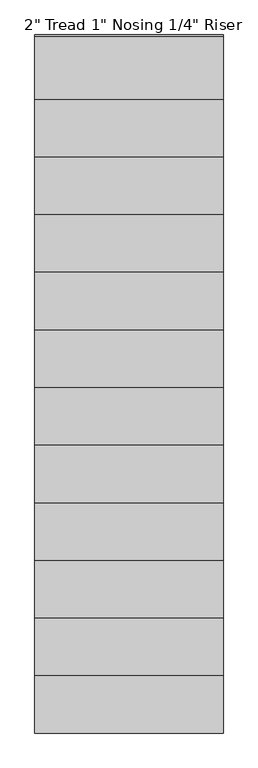
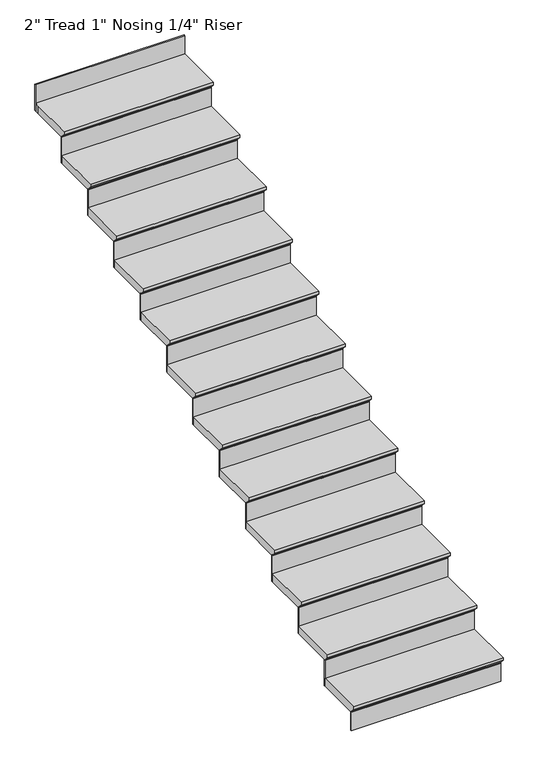
"""IFC4 building model written with IfcOpenShell, lengths in millimetres: stair flight geometry."""

from ifc_helpers import new_model, si_unit, origin, place, context, project, spatial, faceted_brep, source, transform, mapped, element, save


def stair_flight_770626d1(model_context):
    return source(origin(), model_context, "Body", "Brep", [
        faceted_brep([(-2703.0415084, 19841.9216096, 28432.9005799), (-2703.0415084, 19841.9216096, 28451.9505799), (-3617.4415084, 19841.9216096, 28451.9505799), (-3617.4415084, 19841.9216096, 28432.9005799), (-2703.0415084, 19867.3216096, 28407.5005799), (-3617.4415084, 19867.3216096, 28407.5005799), (-2703.0415084, 20146.7216096, 28451.9505799), (-3617.4415084, 20146.7216096, 28451.9505799), (-3617.4415084, 19867.3216096, 28401.1505799), (-3617.4415084, 20146.7216096, 28401.1505799), (-2703.0415084, 20146.7216096, 28401.1505799), (-2703.0415084, 19867.3216096, 28401.1505799)], [[[0, 1, 2, 3]], [[4, 0, 3, 5]], [[2, 1, 6, 7]], [[8, 9, 10, 11]], [[2, 7, 9, 8, 5, 3]], [[8, 11, 4, 5]], [[6, 1, 0, 4, 11, 10]], [[7, 6, 10, 9]]]),
        faceted_brep([(-2703.0415084, 19867.3216096, 28401.1505799), (-2703.0415084, 19867.3216096, 28282.6172466), (-2703.0415084, 19873.6716096, 28282.6172466), (-2703.0415084, 19873.6716096, 28401.1505799), (-3617.4415084, 19867.3216096, 28401.1505799), (-3617.4415084, 19873.6716096, 28401.1505799), (-3617.4415084, 19873.6716096, 28282.6172466), (-3617.4415084, 19867.3216096, 28282.6172466)], [[[0, 1, 2, 3]], [[4, 5, 6, 7]], [[1, 0, 4, 7]], [[2, 1, 7, 6]], [[3, 2, 6, 5]], [[0, 3, 5, 4]]]),
        faceted_brep([(-2703.0415084, 20146.7216096, 28570.4839133), (-2703.0415084, 20146.7216096, 28401.1505799), (-2703.0415084, 20153.0716096, 28401.1505799), (-2703.0415084, 20153.0716096, 28570.4839133), (-3617.4415084, 20146.7216096, 28570.4839133), (-3617.4415084, 20153.0716096, 28570.4839133), (-3617.4415084, 20153.0716096, 28401.1505799), (-3617.4415084, 20146.7216096, 28401.1505799)], [[[0, 1, 2, 3]], [[4, 5, 6, 7]], [[1, 0, 4, 7]], [[2, 1, 7, 6]], [[3, 2, 6, 5]], [[0, 3, 5, 4]]]),
        faceted_brep([(-3617.4415084, 20121.3216096, 28621.2839133), (-2703.0415084, 20121.3216096, 28621.2839133), (-2703.0415084, 20426.1216096, 28621.2839133), (-3617.4415084, 20426.1216096, 28621.2839133), (-3617.4415084, 20146.7216096, 28570.4839133), (-3617.4415084, 20426.1216096, 28570.4839133), (-2703.0415084, 20426.1216096, 28570.4839133), (-2703.0415084, 20146.7216096, 28570.4839133), (-3617.4415084, 20146.7216096, 28576.8339133), (-3617.4415084, 20121.3216096, 28602.2339133), (-2703.0415084, 20146.7216096, 28576.8339133), (-2703.0415084, 20121.3216096, 28602.2339133)], [[[0, 1, 2, 3]], [[4, 5, 6, 7]], [[0, 3, 5, 4, 8, 9]], [[4, 7, 10, 8]], [[2, 1, 11, 10, 7, 6]], [[3, 2, 6, 5]], [[11, 1, 0, 9]], [[10, 11, 9, 8]]]),
        faceted_brep([(-2703.0415084, 20426.1216096, 28739.8172466), (-2703.0415084, 20426.1216096, 28570.4839133), (-2703.0415084, 20432.4716096, 28570.4839133), (-2703.0415084, 20432.4716096, 28739.8172466), (-3617.4415084, 20426.1216096, 28739.8172466), (-3617.4415084, 20432.4716096, 28739.8172466), (-3617.4415084, 20432.4716096, 28570.4839133), (-3617.4415084, 20426.1216096, 28570.4839133)], [[[0, 1, 2, 3]], [[4, 5, 6, 7]], [[1, 0, 4, 7]], [[2, 1, 7, 6]], [[3, 2, 6, 5]], [[0, 3, 5, 4]]]),
        faceted_brep([(-3617.4415084, 20400.7216096, 28790.6172466), (-2703.0415084, 20400.7216096, 28790.6172466), (-2703.0415084, 20705.5216096, 28790.6172466), (-3617.4415084, 20705.5216096, 28790.6172466), (-3617.4415084, 20426.1216096, 28739.8172466), (-3617.4415084, 20705.5216096, 28739.8172466), (-2703.0415084, 20705.5216096, 28739.8172466), (-2703.0415084, 20426.1216096, 28739.8172466), (-3617.4415084, 20426.1216096, 28746.1672466), (-3617.4415084, 20400.7216096, 28771.5672466), (-2703.0415084, 20426.1216096, 28746.1672466), (-2703.0415084, 20400.7216096, 28771.5672466)], [[[0, 1, 2, 3]], [[4, 5, 6, 7]], [[0, 3, 5, 4, 8, 9]], [[4, 7, 10, 8]], [[2, 1, 11, 10, 7, 6]], [[3, 2, 6, 5]], [[11, 1, 0, 9]], [[10, 11, 9, 8]]]),
        faceted_brep([(-2703.0415084, 20705.5216096, 28909.1505799), (-2703.0415084, 20705.5216096, 28739.8172466), (-2703.0415084, 20711.8716096, 28739.8172466), (-2703.0415084, 20711.8716096, 28909.1505799), (-3617.4415084, 20705.5216096, 28909.1505799), (-3617.4415084, 20711.8716096, 28909.1505799), (-3617.4415084, 20711.8716096, 28739.8172466), (-3617.4415084, 20705.5216096, 28739.8172466)], [[[0, 1, 2, 3]], [[4, 5, 6, 7]], [[1, 0, 4, 7]], [[2, 1, 7, 6]], [[3, 2, 6, 5]], [[0, 3, 5, 4]]]),
        faceted_brep([(-3617.4415084, 20680.1216096, 28959.9505799), (-2703.0415084, 20680.1216096, 28959.9505799), (-2703.0415084, 20984.9216096, 28959.9505799), (-3617.4415084, 20984.9216096, 28959.9505799), (-3617.4415084, 20705.5216096, 28909.1505799), (-3617.4415084, 20984.9216096, 28909.1505799), (-2703.0415084, 20984.9216096, 28909.1505799), (-2703.0415084, 20705.5216096, 28909.1505799), (-3617.4415084, 20705.5216096, 28915.5005799), (-3617.4415084, 20680.1216096, 28940.9005799), (-2703.0415084, 20705.5216096, 28915.5005799), (-2703.0415084, 20680.1216096, 28940.9005799)], [[[0, 1, 2, 3]], [[4, 5, 6, 7]], [[0, 3, 5, 4, 8, 9]], [[4, 7, 10, 8]], [[2, 1, 11, 10, 7, 6]], [[3, 2, 6, 5]], [[11, 1, 0, 9]], [[10, 11, 9, 8]]]),
        faceted_brep([(-2703.0415084, 20984.9216096, 29078.4839133), (-2703.0415084, 20984.9216096, 28909.1505799), (-2703.0415084, 20991.2716096, 28909.1505799), (-2703.0415084, 20991.2716096, 29078.4839133), (-3617.4415084, 20984.9216096, 29078.4839133), (-3617.4415084, 20991.2716096, 29078.4839133), (-3617.4415084, 20991.2716096, 28909.1505799), (-3617.4415084, 20984.9216096, 28909.1505799)], [[[0, 1, 2, 3]], [[4, 5, 6, 7]], [[1, 0, 4, 7]], [[2, 1, 7, 6]], [[3, 2, 6, 5]], [[0, 3, 5, 4]]]),
        faceted_brep([(-3617.4415084, 20959.5216096, 29129.2839133), (-2703.0415084, 20959.5216096, 29129.2839133), (-2703.0415084, 21264.3216096, 29129.2839133), (-3617.4415084, 21264.3216096, 29129.2839133), (-3617.4415084, 20984.9216096, 29078.4839133), (-3617.4415084, 21264.3216096, 29078.4839133), (-2703.0415084, 21264.3216096, 29078.4839133), (-2703.0415084, 20984.9216096, 29078.4839133), (-3617.4415084, 20984.9216096, 29084.8339133), (-3617.4415084, 20959.5216096, 29110.2339133), (-2703.0415084, 20984.9216096, 29084.8339133), (-2703.0415084, 20959.5216096, 29110.2339133)], [[[0, 1, 2, 3]], [[4, 5, 6, 7]], [[0, 3, 5, 4, 8, 9]], [[4, 7, 10, 8]], [[2, 1, 11, 10, 7, 6]], [[3, 2, 6, 5]], [[11, 1, 0, 9]], [[10, 11, 9, 8]]]),
        faceted_brep([(-2703.0415084, 21264.3216096, 29247.8172466), (-2703.0415084, 21264.3216096, 29078.4839133), (-2703.0415084, 21270.6716096, 29078.4839133), (-2703.0415084, 21270.6716096, 29247.8172466), (-3617.4415084, 21264.3216096, 29247.8172466), (-3617.4415084, 21270.6716096, 29247.8172466), (-3617.4415084, 21270.6716096, 29078.4839133), (-3617.4415084, 21264.3216096, 29078.4839133)], [[[0, 1, 2, 3]], [[4, 5, 6, 7]], [[1, 0, 4, 7]], [[2, 1, 7, 6]], [[3, 2, 6, 5]], [[0, 3, 5, 4]]]),
        faceted_brep([(-3617.4415084, 21238.9216096, 29298.6172466), (-2703.0415084, 21238.9216096, 29298.6172466), (-2703.0415084, 21543.7216096, 29298.6172466), (-3617.4415084, 21543.7216096, 29298.6172466), (-3617.4415084, 21264.3216096, 29247.8172466), (-3617.4415084, 21543.7216096, 29247.8172466), (-2703.0415084, 21543.7216096, 29247.8172466), (-2703.0415084, 21264.3216096, 29247.8172466), (-3617.4415084, 21264.3216096, 29254.1672466), (-3617.4415084, 21238.9216096, 29279.5672466), (-2703.0415084, 21264.3216096, 29254.1672466), (-2703.0415084, 21238.9216096, 29279.5672466)], [[[0, 1, 2, 3]], [[4, 5, 6, 7]], [[0, 3, 5, 4, 8, 9]], [[4, 7, 10, 8]], [[2, 1, 11, 10, 7, 6]], [[3, 2, 6, 5]], [[11, 1, 0, 9]], [[10, 11, 9, 8]]]),
        faceted_brep([(-2703.0415084, 21543.7216096, 29417.1505799), (-2703.0415084, 21543.7216096, 29247.8172466), (-2703.0415084, 21550.0716096, 29247.8172466), (-2703.0415084, 21550.0716096, 29417.1505799), (-3617.4415084, 21543.7216096, 29417.1505799), (-3617.4415084, 21550.0716096, 29417.1505799), (-3617.4415084, 21550.0716096, 29247.8172466), (-3617.4415084, 21543.7216096, 29247.8172466)], [[[0, 1, 2, 3]], [[4, 5, 6, 7]], [[1, 0, 4, 7]], [[2, 1, 7, 6]], [[3, 2, 6, 5]], [[0, 3, 5, 4]]]),
        faceted_brep([(-3617.4415084, 21518.3216096, 29467.9505799), (-2703.0415084, 21518.3216096, 29467.9505799), (-2703.0415084, 21823.1216096, 29467.9505799), (-3617.4415084, 21823.1216096, 29467.9505799), (-3617.4415084, 21543.7216096, 29417.1505799), (-3617.4415084, 21823.1216096, 29417.1505799), (-2703.0415084, 21823.1216096, 29417.1505799), (-2703.0415084, 21543.7216096, 29417.1505799), (-3617.4415084, 21543.7216096, 29423.5005799), (-3617.4415084, 21518.3216096, 29448.9005799), (-2703.0415084, 21543.7216096, 29423.5005799), (-2703.0415084, 21518.3216096, 29448.9005799)], [[[0, 1, 2, 3]], [[4, 5, 6, 7]], [[0, 3, 5, 4, 8, 9]], [[4, 7, 10, 8]], [[2, 1, 11, 10, 7, 6]], [[3, 2, 6, 5]], [[11, 1, 0, 9]], [[10, 11, 9, 8]]]),
        faceted_brep([(-2703.0415084, 21823.1216096, 29586.4839133), (-2703.0415084, 21823.1216096, 29417.1505799), (-2703.0415084, 21829.4716096, 29417.1505799), (-2703.0415084, 21829.4716096, 29586.4839133), (-3617.4415084, 21823.1216096, 29586.4839133), (-3617.4415084, 21829.4716096, 29586.4839133), (-3617.4415084, 21829.4716096, 29417.1505799), (-3617.4415084, 21823.1216096, 29417.1505799)], [[[0, 1, 2, 3]], [[4, 5, 6, 7]], [[1, 0, 4, 7]], [[2, 1, 7, 6]], [[3, 2, 6, 5]], [[0, 3, 5, 4]]]),
        faceted_brep([(-3617.4415084, 21797.7216096, 29637.2839133), (-2703.0415084, 21797.7216096, 29637.2839133), (-2703.0415084, 22102.5216096, 29637.2839133), (-3617.4415084, 22102.5216096, 29637.2839133), (-3617.4415084, 21823.1216096, 29586.4839133), (-3617.4415084, 22102.5216096, 29586.4839133), (-2703.0415084, 22102.5216096, 29586.4839133), (-2703.0415084, 21823.1216096, 29586.4839133), (-3617.4415084, 21823.1216096, 29592.8339133), (-3617.4415084, 21797.7216096, 29618.2339133), (-2703.0415084, 21823.1216096, 29592.8339133), (-2703.0415084, 21797.7216096, 29618.2339133)], [[[0, 1, 2, 3]], [[4, 5, 6, 7]], [[0, 3, 5, 4, 8, 9]], [[4, 7, 10, 8]], [[2, 1, 11, 10, 7, 6]], [[3, 2, 6, 5]], [[11, 1, 0, 9]], [[10, 11, 9, 8]]]),
        faceted_brep([(-2703.0415084, 22102.5216096, 29755.8172466), (-2703.0415084, 22102.5216096, 29586.4839133), (-2703.0415084, 22108.8716096, 29586.4839133), (-2703.0415084, 22108.8716096, 29755.8172466), (-3617.4415084, 22102.5216096, 29755.8172466), (-3617.4415084, 22108.8716096, 29755.8172466), (-3617.4415084, 22108.8716096, 29586.4839133), (-3617.4415084, 22102.5216096, 29586.4839133)], [[[0, 1, 2, 3]], [[4, 5, 6, 7]], [[1, 0, 4, 7]], [[2, 1, 7, 6]], [[3, 2, 6, 5]], [[0, 3, 5, 4]]]),
        faceted_brep([(-3617.4415084, 22077.1216096, 29806.6172466), (-2703.0415084, 22077.1216096, 29806.6172466), (-2703.0415084, 22381.9216096, 29806.6172466), (-3617.4415084, 22381.9216096, 29806.6172466), (-3617.4415084, 22102.5216096, 29755.8172466), (-3617.4415084, 22381.9216096, 29755.8172466), (-2703.0415084, 22381.9216096, 29755.8172466), (-2703.0415084, 22102.5216096, 29755.8172466), (-3617.4415084, 22102.5216096, 29762.1672466), (-3617.4415084, 22077.1216096, 29787.5672466), (-2703.0415084, 22102.5216096, 29762.1672466), (-2703.0415084, 22077.1216096, 29787.5672466)], [[[0, 1, 2, 3]], [[4, 5, 6, 7]], [[0, 3, 5, 4, 8, 9]], [[4, 7, 10, 8]], [[2, 1, 11, 10, 7, 6]], [[3, 2, 6, 5]], [[11, 1, 0, 9]], [[10, 11, 9, 8]]]),
        faceted_brep([(-2703.0415084, 22381.9216096, 29925.1505799), (-2703.0415084, 22381.9216096, 29755.8172466), (-2703.0415084, 22388.2716096, 29755.8172466), (-2703.0415084, 22388.2716096, 29925.1505799), (-3617.4415084, 22381.9216096, 29925.1505799), (-3617.4415084, 22388.2716096, 29925.1505799), (-3617.4415084, 22388.2716096, 29755.8172466), (-3617.4415084, 22381.9216096, 29755.8172466)], [[[0, 1, 2, 3]], [[4, 5, 6, 7]], [[1, 0, 4, 7]], [[2, 1, 7, 6]], [[3, 2, 6, 5]], [[0, 3, 5, 4]]]),
        faceted_brep([(-3617.4415084, 22356.5216096, 29975.9505799), (-2703.0415084, 22356.5216096, 29975.9505799), (-2703.0415084, 22661.3216096, 29975.9505799), (-3617.4415084, 22661.3216096, 29975.9505799), (-3617.4415084, 22381.9216096, 29925.1505799), (-3617.4415084, 22661.3216096, 29925.1505799), (-2703.0415084, 22661.3216096, 29925.1505799), (-2703.0415084, 22381.9216096, 29925.1505799), (-3617.4415084, 22381.9216096, 29931.5005799), (-3617.4415084, 22356.5216096, 29956.9005799), (-2703.0415084, 22381.9216096, 29931.5005799), (-2703.0415084, 22356.5216096, 29956.9005799)], [[[0, 1, 2, 3]], [[4, 5, 6, 7]], [[0, 3, 5, 4, 8, 9]], [[4, 7, 10, 8]], [[2, 1, 11, 10, 7, 6]], [[3, 2, 6, 5]], [[11, 1, 0, 9]], [[10, 11, 9, 8]]]),
        faceted_brep([(-2703.0415084, 22661.3216096, 30094.4839133), (-2703.0415084, 22661.3216096, 29925.1505799), (-2703.0415084, 22667.6716096, 29925.1505799), (-2703.0415084, 22667.6716096, 30094.4839133), (-3617.4415084, 22661.3216096, 30094.4839133), (-3617.4415084, 22667.6716096, 30094.4839133), (-3617.4415084, 22667.6716096, 29925.1505799), (-3617.4415084, 22661.3216096, 29925.1505799)], [[[0, 1, 2, 3]], [[4, 5, 6, 7]], [[1, 0, 4, 7]], [[2, 1, 7, 6]], [[3, 2, 6, 5]], [[0, 3, 5, 4]]]),
        faceted_brep([(-3617.4415084, 22635.9216096, 30145.2839133), (-2703.0415084, 22635.9216096, 30145.2839133), (-2703.0415084, 22940.7216096, 30145.2839133), (-3617.4415084, 22940.7216096, 30145.2839133), (-3617.4415084, 22661.3216096, 30094.4839133), (-3617.4415084, 22940.7216096, 30094.4839133), (-2703.0415084, 22940.7216096, 30094.4839133), (-2703.0415084, 22661.3216096, 30094.4839133), (-3617.4415084, 22661.3216096, 30100.8339133), (-3617.4415084, 22635.9216096, 30126.2339133), (-2703.0415084, 22661.3216096, 30100.8339133), (-2703.0415084, 22635.9216096, 30126.2339133)], [[[0, 1, 2, 3]], [[4, 5, 6, 7]], [[0, 3, 5, 4, 8, 9]], [[4, 7, 10, 8]], [[2, 1, 11, 10, 7, 6]], [[3, 2, 6, 5]], [[11, 1, 0, 9]], [[10, 11, 9, 8]]]),
        faceted_brep([(-2703.0415084, 23220.1216096, 30433.1505799), (-2703.0415084, 23220.1216096, 30263.8172466), (-2703.0415084, 23226.4716096, 30263.8172466), (-2703.0415084, 23226.4716096, 30433.1505799), (-3617.4415084, 23220.1216096, 30433.1505799), (-3617.4415084, 23226.4716096, 30433.1505799), (-3617.4415084, 23226.4716096, 30263.8172466), (-3617.4415084, 23220.1216096, 30263.8172466)], [[[0, 1, 2, 3]], [[4, 5, 6, 7]], [[1, 0, 4, 7]], [[2, 1, 7, 6]], [[3, 2, 6, 5]], [[0, 3, 5, 4]]]),
        faceted_brep([(-2703.0415084, 22940.7216096, 30263.8172466), (-2703.0415084, 22940.7216096, 30094.4839133), (-2703.0415084, 22947.0716096, 30094.4839133), (-2703.0415084, 22947.0716096, 30263.8172466), (-3617.4415084, 22940.7216096, 30263.8172466), (-3617.4415084, 22947.0716096, 30263.8172466), (-3617.4415084, 22947.0716096, 30094.4839133), (-3617.4415084, 22940.7216096, 30094.4839133)], [[[0, 1, 2, 3]], [[4, 5, 6, 7]], [[1, 0, 4, 7]], [[2, 1, 7, 6]], [[3, 2, 6, 5]], [[0, 3, 5, 4]]]),
        faceted_brep([(-3617.4415084, 23220.1216096, 30314.6172466), (-3617.4415084, 23194.7216096, 30314.6172466), (-3617.4415084, 22915.3216096, 30314.6172466), (-2703.0415084, 22915.3216096, 30314.6172466), (-2703.0415084, 23220.1216096, 30314.6172466), (-3617.4415084, 23194.7216096, 30263.8172466), (-3617.4415084, 23220.1216096, 30263.8172466), (-2703.0415084, 23220.1216096, 30263.8172466), (-2703.0415084, 22940.7216096, 30263.8172466), (-3617.4415084, 22940.7216096, 30263.8172466), (-3617.4415084, 22940.7216096, 30270.1672466), (-3617.4415084, 22915.3216096, 30295.5672466), (-2703.0415084, 22940.7216096, 30270.1672466), (-2703.0415084, 22915.3216096, 30295.5672466)], [[[0, 1, 2, 3, 4]], [[5, 6, 7, 8, 9]], [[1, 0, 6, 5]], [[2, 1, 5, 9, 10, 11]], [[9, 8, 12, 10]], [[4, 3, 13, 12, 8, 7]], [[0, 4, 7, 6]], [[13, 3, 2, 11]], [[12, 13, 11, 10]]]),
    ])


if __name__ == "__main__":
    model = new_model("IFC4")
    model_context = context("Model", 3, world=origin())
    ifc_project = project(units=[si_unit("LENGTHUNIT", "METRE", prefix="MILLI")], contexts=[model_context])
    site = spatial("IfcSite", under=ifc_project)
    building = spatial("IfcBuilding", under=site)
    placement = place(None, origin())
    stair_flight_shape = stair_flight_770626d1(model_context)
    element("IfcStairFlight", 1, ObjectType="2\" Tread 1\" Nosing 1/4\" Riser", at=placement, inside=building, context=model_context, shape_type="MappedRepresentation", body=[
        mapped(stair_flight_shape, transform((0.0, 0.0, 0.0), x_axis=(1.0, 0.0, 0.0), y_axis=(0.0, 1.0, 0.0), z_axis=(0.0, 0.0, 1.0))),
    ])
    save(model, "model.ifc")
